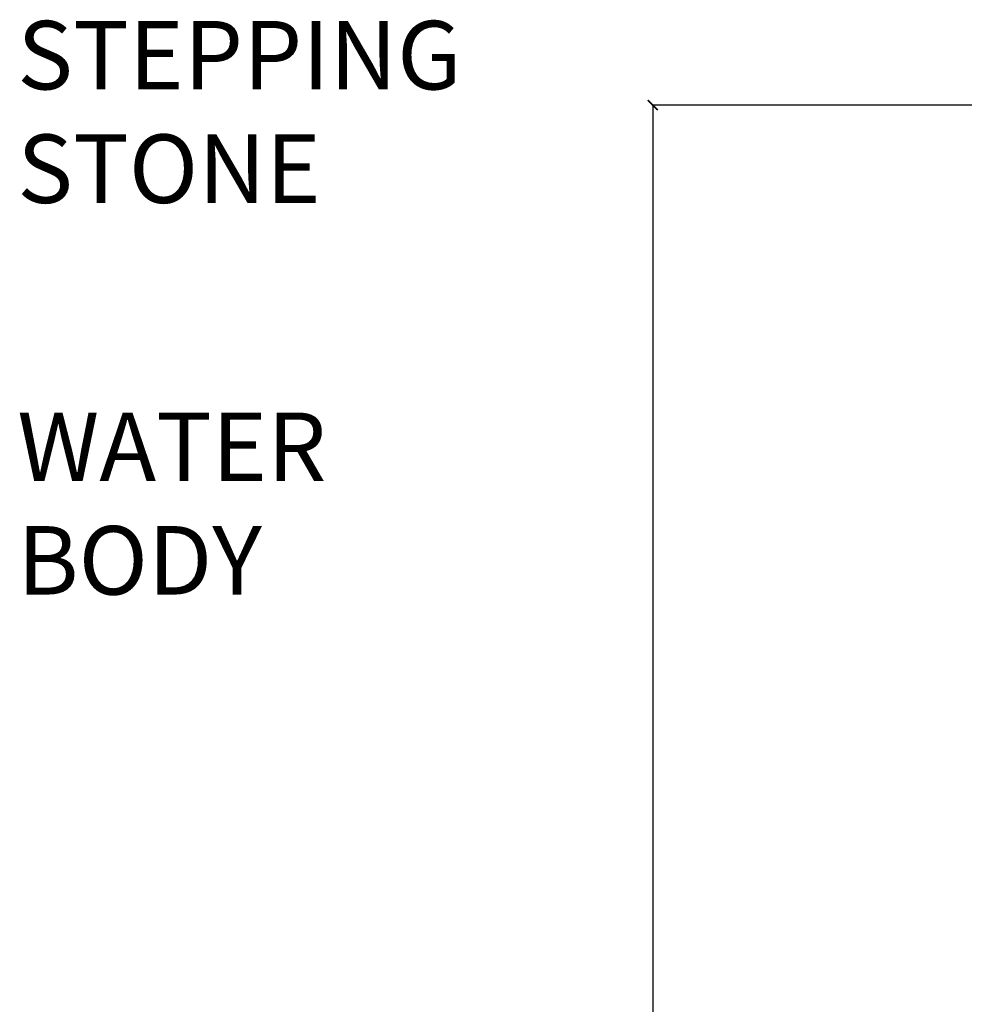
# Model space of a CAD drawing. Units: inches. Extents: x 1704 to 6393, y -157 to 1172.
# Tile 43 of 122: x 1704 to 1892, y 716 to 912. Entities that reach past the tile are written whole.
import ezdxf

# ---------------------------------------------------------------- set-up
doc = ezdxf.new("R2010")
doc.units = ezdxf.units.IN
doc.header["$MEASUREMENT"] = 0
doc.layers.add('A-ANNO-DIMS', color=7, linetype='Continuous', lineweight=13)
doc.layers.add('A-AREA-IDEN', color=7, linetype='Continuous', lineweight=18)
doc.styles.get("Standard").update_dxf_attribs({"font": 'arial.ttf'})
doc.dimstyles.get("Standard").update_dxf_attribs({"dimtxt": 6, "dimasz": 2, "dimexe": 0.18, "dimexo": 0.0625, "dimgap": 0.09, "dimtad": 0, "dimtih": 1, "dimtoh": 1, "dimdec": 1, "dimzin": 0, "dimdsep": 46, "dimlunit": 3, "dimtxsty": 'Standard', "dimblk": 'ARCHTICK', "dimcen": 0.09, "dimadec": 0, "dimazin": 0, "dimtfac": 1, "dimtdec": 1, "dimtofl": 0, "dimtmove": 0, "dimatfit": 3, "dimfxl": 1, "dimtolj": 1, "dimtzin": 0, "dimarcsym": 0})

# ---------------------------------------------------------------- blocks, each defined once
blk = doc.blocks.new('_ArchTick')
at = {"color": 0, "linetype": 'ByBlock', "const_width": 0.15}
blk.add_lwpolyline([(-0.5, -0.5), (0.5, 0.5)], dxfattribs=at)
blk = doc.blocks.new('*D93')
at = {"layer": 'A-ANNO-DIMS', "color": 0, "lineweight": -2, "transparency": 16777216}
for p, q in [((2605.29, 895.21), (1829.7, 895.21)), ((1829.88, 895.21), (1829.88, 495.87)), ((1829.88, 90.21), (1829.88, 489.56)), ((2605.29, 90.21), (1829.7, 90.21))]:
    blk.add_line(p, q, dxfattribs=at)
at = {"layer": 'Defpoints', "color": 0, "lineweight": -3, "transparency": 16777216}
for p in [(2605.35, 895.21), (1829.88, 90.21), (2605.35, 90.21)]:
    blk.add_point(p, dxfattribs=at)
at = {"layer": 'A-ANNO-DIMS', "color": 0, "lineweight": -2, "transparency": 16777216, "xscale": 2, "yscale": 2, "zscale": 2}
for p, rotation in [((1829.88, 895.21), 90), ((1829.88, 90.21), 270)]:
    blk.add_blockref('_ArchTick', p, dxfattribs=dict(at, rotation=rotation))
at = {"layer": 'A-ANNO-DIMS', "color": 0, "transparency": 16777216, "insert": (1829.88, 492.71), "char_height": 6, "attachment_point": 5}
blk.add_mtext('\\A1;805', dxfattribs=at)

msp = doc.modelspace()

# ---------------------------------------------------------------- texts
at = {"layer": 'A-AREA-IDEN'}
for s, p in [('STEPPING', (1703.067, 898.338)), ('STONE', (1703.067, 875.675)), ('WATER', (1703.067, 820.194)), ('BODY', (1703.067, 797.53))]:
    msp.add_text(s, height=13.6672, dxfattribs=at).set_placement(p)

# ---------------------------------------------------------------- dimensions: what is measured, and where the dimension line sits
at = {"layer": 'A-ANNO-DIMS'}
dim = msp.add_linear_dim(base=(1829.878, 90.213), p1=(2605.349, 895.213), p2=(2605.349, 90.213), angle=90, dimstyle='Standard', override={"dimdec": 0, "dimlfac": 1, "dimrnd": 0, "dimzin": 0, "dimdsep": 46, "dimlunit": 2}, dxfattribs=at)
dim.commit()
dim.dimension.update_dxf_attribs({"geometry": '*D93', "text_midpoint": (1829.878, 492.713)})

doc.saveas('drawing.dxf')
